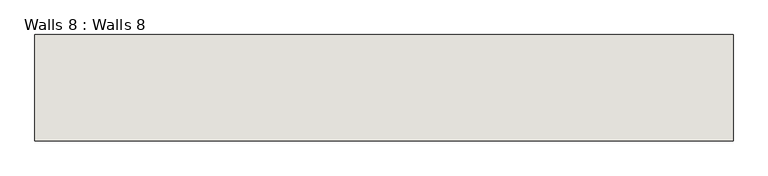
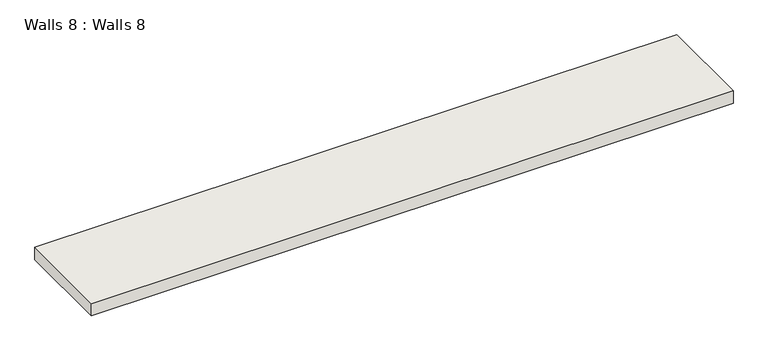
"""IFC4 building model written with IfcOpenShell, lengths in millimetres: wall geometry, Walls 8 : Walls 8."""

from ifc_helpers import new_model, si_unit, frame, origin, place, context, project, spatial, polyline, outline, extrude, source, transform, mapped, element, save


def walls_8_walls_8_172a5026(model_context):
    return source(origin(), model_context, "Body", "SweptSolid", [
        extrude(outline(polyline([(-15798.6897324, -3824.3180898), (-15798.6897324, -3390.9180898), (-12954.6289001, -3390.9180898), (-12954.6289001, -3824.3180898), (-15798.6897324, -3824.3180898)])), frame((0.0, 0.0, 3830.5245478), z_axis=(0.0, 0.0, 1.0), x_axis=(1.0, 0.0, 0.0)), (0.0, 0.0, 1.0), 56.7782892),
    ])


if __name__ == "__main__":
    model = new_model("IFC4")
    model_context = context("Model", 3, world=origin())
    ifc_project = project(units=[si_unit("LENGTHUNIT", "METRE", prefix="MILLI")], contexts=[model_context])
    site = spatial("IfcSite", under=ifc_project)
    building = spatial("IfcBuilding", under=site)
    placement = place(None, origin())
    walls_8_walls_8_shape = walls_8_walls_8_172a5026(model_context)
    element("IfcWall", 1, ObjectType="Walls 8 : Walls 8", at=placement, inside=building, context=model_context, shape_type="MappedRepresentation", body=[
        mapped(walls_8_walls_8_shape, transform((0.0, 0.0, 0.0), x_axis=(1.0, 0.0, 0.0), y_axis=(0.0, 1.0, 0.0), z_axis=(0.0, 0.0, 1.0))),
    ])
    save(model, "model.ifc")

# Revit data of these elements
# Element 1 (IfcWall, "Walls 8 : Walls 8")
#   Materials on its faces: "Default Wall"
# Materials
#   "Default Wall": colour RGB 80 80 80, transparency 0
